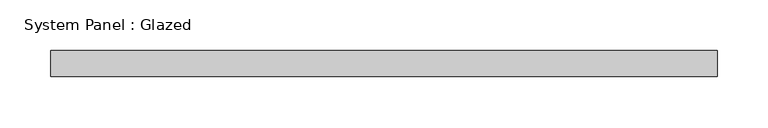
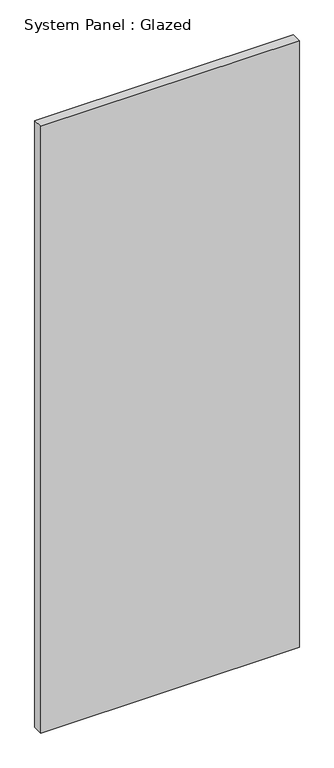
"""IFC4 building model written with IfcOpenShell, lengths in millimetres: plate geometry, System Panel : Glazed."""

from ifc_helpers import new_model, si_unit, origin, origin_with_axes, place, context, project, spatial, polyline, outline, extrude, source, transform, mapped, element, save


def system_panel_glazed_762caeb2(model_context):
    return source(origin(), model_context, "Body", "SweptSolid", [
        extrude(outline(polyline([(327.025, 19.05), (-327.025, 19.05), (-327.025, 44.45), (327.025, 44.45), (327.025, 19.05)])), origin_with_axes(), (0.0, 0.0, 1.0), 1620.5125275),
    ])


if __name__ == "__main__":
    model = new_model("IFC4")
    model_context = context("Model", 3, world=origin())
    ifc_project = project(units=[si_unit("LENGTHUNIT", "METRE", prefix="MILLI")], contexts=[model_context])
    site = spatial("IfcSite", under=ifc_project)
    building = spatial("IfcBuilding", under=site)
    placement = place(None, origin())
    system_panel_glazed_shape = system_panel_glazed_762caeb2(model_context)
    element("IfcPlate", 1, ObjectType="System Panel : Glazed", at=placement, inside=building, context=model_context, shape_type="MappedRepresentation", body=[
        mapped(system_panel_glazed_shape, transform((0.0, 0.0, 0.0), x_axis=(1.0, 0.0, 0.0), y_axis=(0.0, 1.0, 0.0), z_axis=(0.0, 0.0, 1.0))),
    ])
    save(model, "model.ifc")

# Revit data of these elements
# Type "System Panel : Glazed"
#   Construction Type Id = "GSP4R"
#   Analytic Construction = "1/8 in Pilkington single glazing"
#   Visual Light Transmittance = 0.9
#   Solar Heat Gain Coefficient = 0.86
#   Heat Transfer Coefficient (U) = 1.18115 BTU/(h·ft²·°F)
#   Define Thermal Properties by = 1
# Element 1 (IfcPlate, "System Panel : Glazed")
#   Materials on its faces: "Glass"
# Materials
#   "Glass": class "Glass", colour RGB 0 128 192, transparency 0.75, Description = "Soda Lime Glass", Cost = 0
